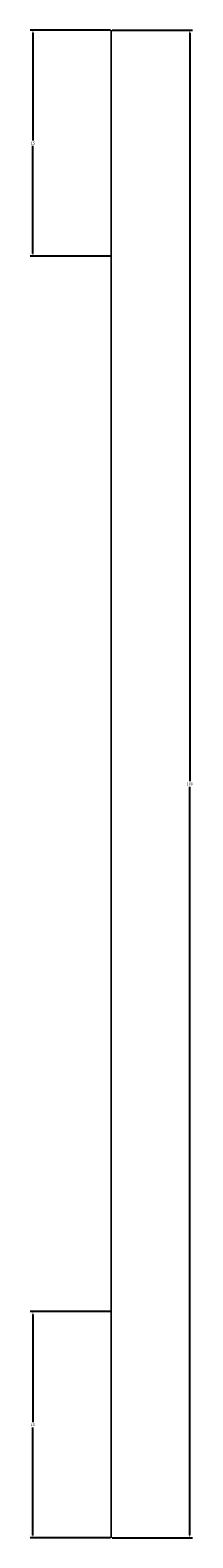
# Model space of a CAD drawing. Units: millimetres. Extents: x -5 to 2707, y 665 to 1247.
# Tile 1 of 3: x -5 to 5, y 977 to 1077. Entities that reach past the tile are written whole.
import ezdxf

# ---------------------------------------------------------------- set-up
doc = ezdxf.new("R2010")
doc.units = ezdxf.units.MM
doc.layers.add('M-CONS', color=7, linetype='Continuous', lineweight=18)
doc.layers.add('M-DIMS', color=2, linetype='Continuous', lineweight=18)
doc.styles.get("Standard").update_dxf_attribs({"font": 'arial.ttf'})
doc.dimstyles.get("Standard").update_dxf_attribs({"dimtxt": 0.18, "dimasz": 0.18, "dimexe": 0.18, "dimexo": 0.0625, "dimgap": 0.09, "dimtad": 0, "dimtih": 1, "dimtoh": 1, "dimdec": 4, "dimzin": 0, "dimdsep": 46, "dimtxsty": 'Standard', "dimcen": 0.09, "dimadec": 0, "dimazin": 0, "dimtfac": 1, "dimtdec": 4, "dimtofl": 0, "dimtmove": 0, "dimatfit": 3, "dimfxl": 1, "dimtolj": 1, "dimtzin": 0, "dimarcsym": 0})

# ---------------------------------------------------------------- blocks, each defined once
blk = doc.blocks.new('*D12')
at = {"layer": 'Defpoints', "color": 0, "transparency": 16777216}
for p in [(0, 1076.91), (5.2, 1076.91), (0, 976.91)]:
    blk.add_point(p, dxfattribs=at)
at = {"layer": 'M-DIMS', "color": 0, "lineweight": -2, "transparency": 16777216}
for p, q in [((0.06, 1076.91), (5.38, 1076.91)), ((5.2, 1076.73), (5.2, 1027.09)), ((5.2, 977.09), (5.2, 1026.73)), ((0.06, 976.91), (5.38, 976.91))]:
    blk.add_line(p, q, dxfattribs=at)
at = {"layer": 'M-DIMS', "color": 0, "transparency": 16777216}
for points in [[(5.17, 1076.73), (5.23, 1076.73), (5.2, 1076.91)], [(5.17, 977.09), (5.23, 977.09), (5.2, 976.91)]]:
    blk.add_solid(points, dxfattribs=at)
at = {"layer": 'M-DIMS', "color": 0, "transparency": 16777216, "insert": (5.2, 1026.91), "char_height": 0.18, "attachment_point": 5}
blk.add_mtext('\\A1;100', dxfattribs=at)
blk = doc.blocks.new('*D13')
at = {"layer": 'Defpoints', "color": 0, "transparency": 16777216}
for p in [(-5.2, 991.91), (0, 991.91), (0, 976.91)]:
    blk.add_point(p, dxfattribs=at)
at = {"layer": 'M-DIMS', "color": 0, "lineweight": -2, "transparency": 16777216}
for p, q in [((-0.06, 991.91), (-5.38, 991.91)), ((-5.2, 991.73), (-5.2, 984.59)), ((-5.2, 977.09), (-5.2, 984.23)), ((-0.06, 976.91), (-5.38, 976.91))]:
    blk.add_line(p, q, dxfattribs=at)
at = {"layer": 'M-DIMS', "color": 0, "transparency": 16777216}
for points in [[(-5.23, 991.73), (-5.17, 991.73), (-5.2, 991.91)], [(-5.23, 977.09), (-5.17, 977.09), (-5.2, 976.91)]]:
    blk.add_solid(points, dxfattribs=at)
at = {"layer": 'M-DIMS', "color": 0, "transparency": 16777216, "insert": (-5.2, 984.41), "char_height": 0.18, "attachment_point": 5}
blk.add_mtext('\\A1;15', dxfattribs=at)
blk = doc.blocks.new('*D14')
at = {"layer": 'Defpoints', "color": 0, "transparency": 16777216}
for p in [(0, 1076.91), (-5.2, 1061.91), (0, 1061.91)]:
    blk.add_point(p, dxfattribs=at)
at = {"layer": 'M-DIMS', "color": 0, "lineweight": -2, "transparency": 16777216}
for p, q in [((-0.06, 1076.91), (-5.38, 1076.91)), ((-5.2, 1076.73), (-5.2, 1069.59)), ((-5.2, 1062.09), (-5.2, 1069.23)), ((-0.06, 1061.91), (-5.38, 1061.91))]:
    blk.add_line(p, q, dxfattribs=at)
at = {"layer": 'M-DIMS', "color": 0, "transparency": 16777216}
for points in [[(-5.23, 1076.73), (-5.17, 1076.73), (-5.2, 1076.91)], [(-5.23, 1062.09), (-5.17, 1062.09), (-5.2, 1061.91)]]:
    blk.add_solid(points, dxfattribs=at)
at = {"layer": 'M-DIMS', "color": 0, "transparency": 16777216, "insert": (-5.2, 1069.41), "char_height": 0.18, "attachment_point": 5}
blk.add_mtext('\\A1;15', dxfattribs=at)

msp = doc.modelspace()

# ---------------------------------------------------------------- linework, layer by layer
at = {"layer": 'M-CONS', "extrusion": (1, 0, 0)}
msp.add_lwpolyline([(1076.9069, -0.8757, 0.41421356), (1061.9069, 14.1243), (991.9069, 14.1243, 0.41421356), (976.9069, -0.8757), (976.9069, -35.8757), (1076.9069, -35.8757)], format="xyb", close=True, dxfattribs=at)

# ---------------------------------------------------------------- dimensions: what is measured, and where the dimension line sits
at = {"layer": 'M-DIMS'}
for base, p1, p2, picture, middle in [((-5.2, 1061.9069), (0, 1076.9069), (0, 1061.9069), '*D14', (-5.2, 1069.4069)), ((5.2, 1076.9069), (0, 976.9069), (0, 1076.9069), '*D12', (5.2, 1026.9069)), ((-5.2, 991.9069), (0, 976.9069), (0, 991.9069), '*D13', (-5.2, 984.4069))]:
    dim = msp.add_linear_dim(base=base, p1=p1, p2=p2, angle=90, dimstyle='Standard', override={"dimdec": 0, "dimlfac": 1, "dimrnd": 0, "dimzin": 0, "dimdsep": 46, "dimlunit": 2}, dxfattribs=at)
    dim.commit()
    dim.dimension.update_dxf_attribs({"geometry": picture, "text_midpoint": middle})

doc.saveas('drawing.dxf')
